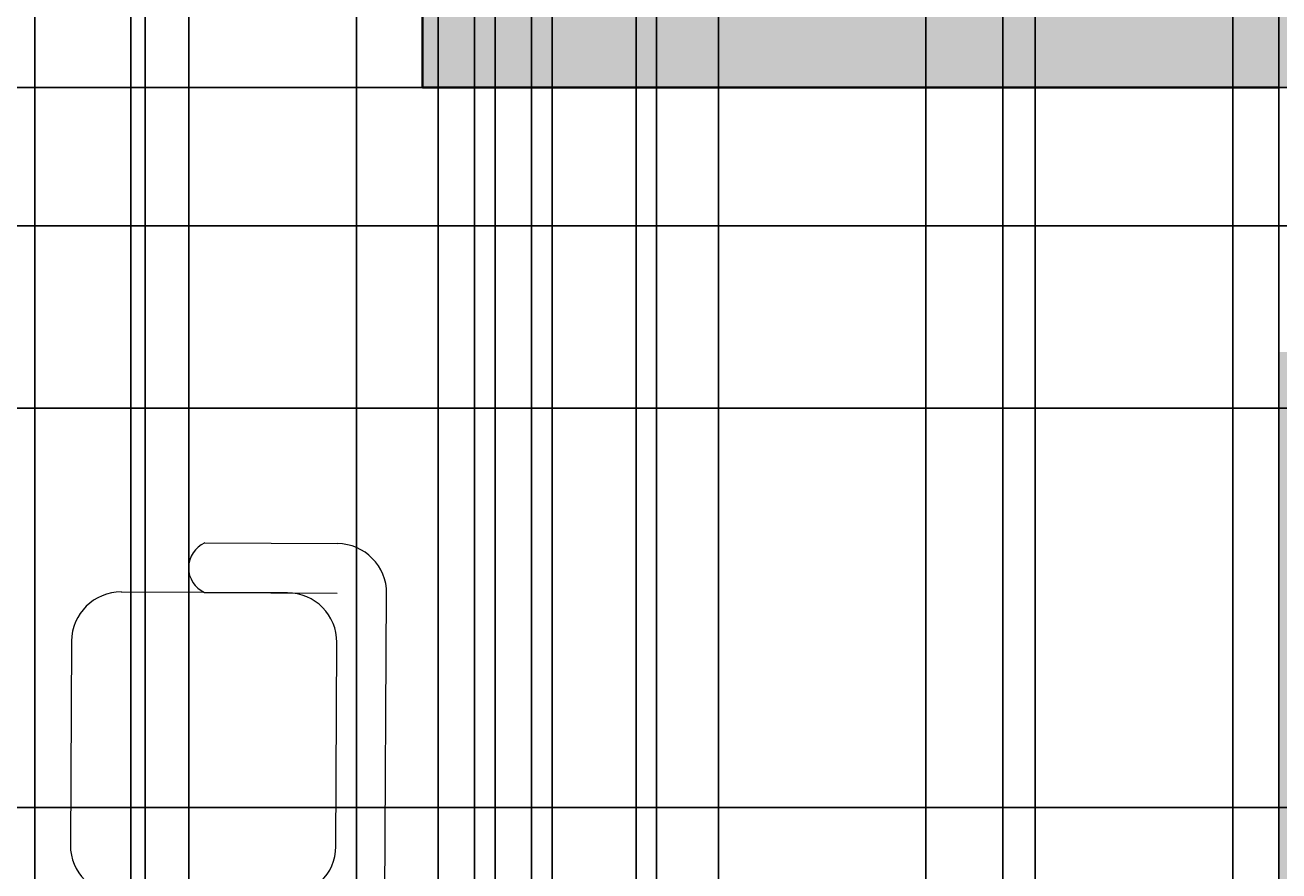
# Model space of a CAD drawing. Units: inches. Extents: x 818 to 1898, y 976 to 2364.
# Tile 37 of 96: x 1391 to 1512, y 1792 to 1873. Entities that reach past the tile are written whole.
import ezdxf

# ---------------------------------------------------------------- set-up
doc = ezdxf.new("R2010")
doc.units = ezdxf.units.IN
doc.header["$LTSCALE"] = 5
doc.header["$MEASUREMENT"] = 0
for name, color, linetype, lineweight in [('A-ANNO-DIMS', 2, 'Continuous', 18), ('A-FURN', 8, 'Continuous', 18), ('A-WALL', 7, 'Continuous', 40)]:
    doc.layers.add(name, color=color, linetype=linetype, lineweight=lineweight)
doc.layers.add('A-WALL-PATT', color=251, linetype='Continuous', lineweight=13, true_color=0x636466)
doc.styles.get("Standard").update_dxf_attribs({"font": 'arial.ttf'})
doc.dimstyles.get("Standard").update_dxf_attribs({"dimtxt": 0.18, "dimasz": 0.18, "dimexe": 0.18, "dimexo": 0.0625, "dimgap": 0.09, "dimtad": 0, "dimtih": 1, "dimtoh": 1, "dimdec": 4, "dimzin": 0, "dimdsep": 46, "dimtxsty": 'Standard', "dimcen": 0.09, "dimadec": 0, "dimazin": 0, "dimtfac": 1, "dimtdec": 4, "dimtofl": 0, "dimtmove": 0, "dimatfit": 3, "dimfxl": 1, "dimtolj": 1, "dimtzin": 0, "dimarcsym": 0})

# ---------------------------------------------------------------- blocks, each defined once
blk = doc.blocks.new('CHAIR-LOUNGE')
for p, q in [((12.94, 38.78), (25.71, 38.71)), ((20.92, 33.97), (4.9, 34.05)), ((12.91, 34.01), (25.69, 33.94)), ((30.3, 4.74), (30.46, 33.92)), ((0.11, 29.31), (0, 9.68)), ((25.56, 9.54), (25.66, 29.17)), ((19.37, 4.79), (3.35, 4.88)), ((4.74, 4.88), (20.76, 4.79)), ((11.36, 4.84), (24.14, 4.77)), ((12.75, 4.84), (25.53, 4.77)), ((12.73, 0.07), (25.5, 0))]:
    blk.add_line(p, q)
for centre, radius, start, end in [((13.99, 36.39), 2.61, 113.7099, 245.6698), ((25.69, 33.94), 4.77, 359.6898, 89.6898), ((4.88, 29.29), 4.77, 89.6898, 179.6898), ((20.89, 29.2), 4.77, 359.6898, 89.6898), ((4.77, 9.65), 4.77, 179.6898, 269.6898), ((20.79, 9.56), 4.77, 269.6898, 359.6898), ((13.7, 2.45), 2.57, 111.7034, 247.6762), ((19.35, 0.03), 4.77, 359.6898, 89.6898), ((25.53, 4.77), 4.77, 269.6898, 359.6898)]:
    blk.add_arc(centre, radius, start, end)
blk = doc.blocks.new('*D61')
at = {"layer": 'A-ANNO-DIMS', "color": 0, "lineweight": -2, "ltscale": 5, "transparency": 16777216}
for p, q in [((1071.73, 1203.03), (1071.73, 2363.87)), ((1071.91, 2363.69), (1250.94, 2363.69)), ((1430.55, 2363.69), (1251.51, 2363.69)), ((1430.73, 1203.03), (1430.73, 2363.87))]:
    blk.add_line(p, q, dxfattribs=at)
at = {"layer": 'A-ANNO-DIMS', "color": 0, "ltscale": 5, "transparency": 16777216}
for points in [[(1071.91, 2363.72), (1071.91, 2363.66), (1071.73, 2363.69)], [(1430.55, 2363.72), (1430.55, 2363.66), (1430.73, 2363.69)]]:
    blk.add_solid(points, dxfattribs=at)
at = {"layer": 'Defpoints', "color": 0, "ltscale": 5, "transparency": 16777216}
for p in [(1430.73, 2363.69), (1071.73, 1202.96), (1430.73, 1202.96)]:
    blk.add_point(p, dxfattribs=at)
at = {"layer": 'A-ANNO-DIMS', "color": 0, "ltscale": 5, "transparency": 16777216, "insert": (1251.23, 2363.69), "char_height": 0.18, "attachment_point": 5}
blk.add_mtext('\\A1;359', dxfattribs=at)
blk = doc.blocks.new('*D64')
at = {"layer": 'A-ANNO-DIMS', "color": 0, "lineweight": -2, "ltscale": 5, "transparency": 16777216}
for p, q in [((1197.73, 1501.14), (1197.73, 2363.87)), ((1197.91, 2363.69), (1313.93, 2363.69)), ((1430.55, 2363.69), (1314.52, 2363.69)), ((1430.73, 1501.14), (1430.73, 2363.87))]:
    blk.add_line(p, q, dxfattribs=at)
at = {"layer": 'A-ANNO-DIMS', "color": 0, "ltscale": 5, "transparency": 16777216}
for points in [[(1197.91, 2363.72), (1197.91, 2363.66), (1197.73, 2363.69)], [(1430.55, 2363.72), (1430.55, 2363.66), (1430.73, 2363.69)]]:
    blk.add_solid(points, dxfattribs=at)
at = {"layer": 'Defpoints', "color": 0, "ltscale": 5, "transparency": 16777216}
for p in [(1430.73, 2363.69), (1197.73, 1501.08), (1430.73, 1501.08)]:
    blk.add_point(p, dxfattribs=at)
at = {"layer": 'A-ANNO-DIMS', "color": 0, "ltscale": 5, "transparency": 16777216, "insert": (1314.23, 2363.69), "char_height": 0.18, "attachment_point": 5}
blk.add_mtext('\\A1;233', dxfattribs=at)
blk = doc.blocks.new('*D85')
at = {"layer": 'A-ANNO-DIMS', "color": 0, "lineweight": -2, "ltscale": 5, "transparency": 16777216}
for p, q in [((1258.79, 2053.08), (1897.92, 2053.08)), ((1897.74, 2052.9), (1897.74, 1876.76)), ((1897.74, 1700.26), (1897.74, 1876.4)), ((1258.79, 1700.08), (1897.92, 1700.08))]:
    blk.add_line(p, q, dxfattribs=at)
at = {"layer": 'A-ANNO-DIMS', "color": 0, "ltscale": 5, "transparency": 16777216}
for points in [[(1897.71, 2052.9), (1897.77, 2052.9), (1897.74, 2053.08)], [(1897.71, 1700.26), (1897.77, 1700.26), (1897.74, 1700.08)]]:
    blk.add_solid(points, dxfattribs=at)
at = {"layer": 'Defpoints', "color": 0, "ltscale": 5, "transparency": 16777216}
for p in [(1258.73, 2053.08), (1897.74, 2053.08), (1258.73, 1700.08)]:
    blk.add_point(p, dxfattribs=at)
at = {"layer": 'A-ANNO-DIMS', "color": 0, "ltscale": 5, "transparency": 16777216, "insert": (1897.74, 1876.58), "char_height": 0.18, "attachment_point": 5}
blk.add_mtext('\\A1;353', dxfattribs=at)
blk = doc.blocks.new('*D98')
at = {"layer": 'A-ANNO-DIMS', "color": 0, "lineweight": -2, "ltscale": 5, "transparency": 16777216}
for p, q in [((1338.54, 1071.12), (1338.54, 2363.87)), ((1338.72, 2363.69), (1364.81, 2363.69)), ((1391.7, 2363.69), (1365.6, 2363.69)), ((1391.88, 1071.12), (1391.88, 2363.87))]:
    blk.add_line(p, q, dxfattribs=at)
at = {"layer": 'A-ANNO-DIMS', "color": 0, "ltscale": 5, "transparency": 16777216}
for points in [[(1338.72, 2363.72), (1338.72, 2363.66), (1338.54, 2363.69)], [(1391.7, 2363.72), (1391.7, 2363.66), (1391.88, 2363.69)]]:
    blk.add_solid(points, dxfattribs=at)
at = {"layer": 'Defpoints', "color": 0, "ltscale": 5, "transparency": 16777216}
for p in [(1391.88, 2363.69), (1338.54, 1071.06), (1391.88, 1071.06)]:
    blk.add_point(p, dxfattribs=at)
at = {"layer": 'A-ANNO-DIMS', "color": 0, "ltscale": 5, "transparency": 16777216, "insert": (1365.21, 2363.69), "char_height": 0.18, "attachment_point": 5}
blk.add_mtext('\\A1;53.33', dxfattribs=at)
blk = doc.blocks.new('*D99')
at = {"layer": 'A-ANNO-DIMS', "color": 0, "lineweight": -2, "ltscale": 5, "transparency": 16777216}
for p, q in [((1391.88, 1071.12), (1391.88, 2363.87)), ((1392.06, 2363.69), (1420.45, 2363.69)), ((1449.64, 2363.69), (1421.24, 2363.69)), ((1449.82, 1071.12), (1449.82, 2363.87))]:
    blk.add_line(p, q, dxfattribs=at)
at = {"layer": 'A-ANNO-DIMS', "color": 0, "ltscale": 5, "transparency": 16777216}
for points in [[(1392.06, 2363.72), (1392.06, 2363.66), (1391.88, 2363.69)], [(1449.64, 2363.72), (1449.64, 2363.66), (1449.82, 2363.69)]]:
    blk.add_solid(points, dxfattribs=at)
at = {"layer": 'Defpoints', "color": 0, "ltscale": 5, "transparency": 16777216}
for p in [(1449.82, 2363.69), (1391.88, 1071.06), (1449.82, 1071.06)]:
    blk.add_point(p, dxfattribs=at)
at = {"layer": 'A-ANNO-DIMS', "color": 0, "ltscale": 5, "transparency": 16777216, "insert": (1420.85, 2363.69), "char_height": 0.18, "attachment_point": 5}
blk.add_mtext('\\A1;57.94', dxfattribs=at)
blk = doc.blocks.new('*D100')
at = {"layer": 'A-ANNO-DIMS', "color": 0, "lineweight": -2, "ltscale": 5, "transparency": 16777216}
for p, q in [((1449.82, 1071.12), (1449.82, 2363.87)), ((1450, 2363.69), (1478.17, 2363.69)), ((1507.12, 2363.69), (1478.95, 2363.69)), ((1507.3, 1071.12), (1507.3, 2363.87))]:
    blk.add_line(p, q, dxfattribs=at)
at = {"layer": 'A-ANNO-DIMS', "color": 0, "ltscale": 5, "transparency": 16777216}
for points in [[(1450, 2363.72), (1450, 2363.66), (1449.82, 2363.69)], [(1507.12, 2363.72), (1507.12, 2363.66), (1507.3, 2363.69)]]:
    blk.add_solid(points, dxfattribs=at)
at = {"layer": 'Defpoints', "color": 0, "ltscale": 5, "transparency": 16777216}
for p in [(1507.3, 2363.69), (1449.82, 1071.06), (1507.3, 1071.06)]:
    blk.add_point(p, dxfattribs=at)
at = {"layer": 'A-ANNO-DIMS', "color": 0, "ltscale": 5, "transparency": 16777216, "insert": (1478.56, 2363.69), "char_height": 0.18, "attachment_point": 5}
blk.add_mtext('\\A1;57.48', dxfattribs=at)
blk = doc.blocks.new('*D101')
at = {"layer": 'A-ANNO-DIMS', "color": 0, "lineweight": -2, "ltscale": 5, "transparency": 16777216}
for p, q in [((1507.3, 1071.12), (1507.3, 2363.87)), ((1507.48, 2363.69), (1536, 2363.69)), ((1565.3, 2363.69), (1536.78, 2363.69)), ((1565.48, 1071.12), (1565.48, 2363.87))]:
    blk.add_line(p, q, dxfattribs=at)
at = {"layer": 'A-ANNO-DIMS', "color": 0, "ltscale": 5, "transparency": 16777216}
for points in [[(1507.48, 2363.72), (1507.48, 2363.66), (1507.3, 2363.69)], [(1565.3, 2363.72), (1565.3, 2363.66), (1565.48, 2363.69)]]:
    blk.add_solid(points, dxfattribs=at)
at = {"layer": 'Defpoints', "color": 0, "ltscale": 5, "transparency": 16777216}
for p in [(1565.48, 2363.69), (1507.3, 1071.06), (1565.48, 1071.06)]:
    blk.add_point(p, dxfattribs=at)
at = {"layer": 'A-ANNO-DIMS', "color": 0, "ltscale": 5, "transparency": 16777216, "insert": (1536.39, 2363.69), "char_height": 0.18, "attachment_point": 5}
blk.add_mtext('\\A1;58.19', dxfattribs=at)
blk = doc.blocks.new('*D120')
at = {"layer": 'A-ANNO-DIMS', "color": 0, "lineweight": -2, "ltscale": 5, "transparency": 16777216}
for p, q in [((1766.29, 1797.72), (818.03, 1797.72)), ((818.21, 1797.54), (818.21, 1757.53)), ((818.21, 1717.17), (818.21, 1757.17)), ((1766.29, 1716.99), (818.03, 1716.99))]:
    blk.add_line(p, q, dxfattribs=at)
at = {"layer": 'A-ANNO-DIMS', "color": 0, "ltscale": 5, "transparency": 16777216}
for points in [[(818.18, 1797.54), (818.24, 1797.54), (818.21, 1797.72)], [(818.18, 1717.17), (818.24, 1717.17), (818.21, 1716.99)]]:
    blk.add_solid(points, dxfattribs=at)
at = {"layer": 'Defpoints', "color": 0, "ltscale": 5, "transparency": 16777216}
for p in [(818.21, 1797.72), (1766.35, 1797.72), (1766.35, 1716.99)]:
    blk.add_point(p, dxfattribs=at)
at = {"layer": 'A-ANNO-DIMS', "color": 0, "ltscale": 5, "transparency": 16777216, "insert": (818.21, 1757.35), "char_height": 0.18, "attachment_point": 5}
blk.add_mtext('\\A1;80.73', dxfattribs=at)
blk = doc.blocks.new('*D121')
at = {"layer": 'A-ANNO-DIMS', "color": 0, "lineweight": -2, "ltscale": 5, "transparency": 16777216}
for p, q in [((1766.29, 1884.2), (818.03, 1884.2)), ((818.21, 1884.02), (818.21, 1841.14)), ((818.21, 1797.9), (818.21, 1840.78)), ((1766.29, 1797.72), (818.03, 1797.72))]:
    blk.add_line(p, q, dxfattribs=at)
at = {"layer": 'A-ANNO-DIMS', "color": 0, "ltscale": 5, "transparency": 16777216}
for points in [[(818.18, 1884.02), (818.24, 1884.02), (818.21, 1884.2)], [(818.18, 1797.9), (818.24, 1797.9), (818.21, 1797.72)]]:
    blk.add_solid(points, dxfattribs=at)
at = {"layer": 'Defpoints', "color": 0, "ltscale": 5, "transparency": 16777216}
for p in [(818.21, 1884.2), (1766.35, 1884.2), (1766.35, 1797.72)]:
    blk.add_point(p, dxfattribs=at)
at = {"layer": 'A-ANNO-DIMS', "color": 0, "ltscale": 5, "transparency": 16777216, "insert": (818.21, 1840.96), "char_height": 0.18, "attachment_point": 5}
blk.add_mtext('\\A1;86.49', dxfattribs=at)
blk = doc.blocks.new('*D162')
at = {"layer": 'A-ANNO-DIMS', "color": 0, "lineweight": -2, "ltscale": 5, "transparency": 16777216}
for p, q in [((1429.16, 1876.08), (818.03, 1876.08)), ((818.21, 1875.9), (818.21, 1871.76)), ((818.21, 1867.26), (818.21, 1871.4)), ((1429.16, 1867.08), (818.03, 1867.08))]:
    blk.add_line(p, q, dxfattribs=at)
at = {"layer": 'A-ANNO-DIMS', "color": 0, "ltscale": 5, "transparency": 16777216}
for points in [[(818.18, 1875.9), (818.24, 1875.9), (818.21, 1876.08)], [(818.18, 1867.26), (818.24, 1867.26), (818.21, 1867.08)]]:
    blk.add_solid(points, dxfattribs=at)
at = {"layer": 'Defpoints', "color": 0, "ltscale": 5, "transparency": 16777216}
for p in [(1429.23, 1876.08), (818.21, 1867.08), (1429.23, 1867.08)]:
    blk.add_point(p, dxfattribs=at)
at = {"layer": 'A-ANNO-DIMS', "color": 0, "ltscale": 5, "transparency": 16777216, "insert": (818.21, 1871.58), "char_height": 0.18, "attachment_point": 5}
blk.add_mtext('\\A1;9', dxfattribs=at)
blk = doc.blocks.new('*D166')
at = {"layer": 'A-ANNO-DIMS', "color": 0, "lineweight": -2, "ltscale": 5, "transparency": 16777216}
for p, q in [((1401.15, 1510.14), (1401.15, 2363.87)), ((1401.33, 2363.69), (1415.54, 2363.69)), ((1430.55, 2363.69), (1416.33, 2363.69)), ((1430.73, 1510.14), (1430.73, 2363.87))]:
    blk.add_line(p, q, dxfattribs=at)
at = {"layer": 'A-ANNO-DIMS', "color": 0, "ltscale": 5, "transparency": 16777216}
for points in [[(1401.33, 2363.72), (1401.33, 2363.66), (1401.15, 2363.69)], [(1430.55, 2363.72), (1430.55, 2363.66), (1430.73, 2363.69)]]:
    blk.add_solid(points, dxfattribs=at)
at = {"layer": 'Defpoints', "color": 0, "ltscale": 5, "transparency": 16777216}
for p in [(1430.73, 2363.69), (1401.15, 1510.08), (1430.73, 1510.08)]:
    blk.add_point(p, dxfattribs=at)
at = {"layer": 'A-ANNO-DIMS', "color": 0, "ltscale": 5, "transparency": 16777216, "insert": (1415.94, 2363.69), "char_height": 0.18, "attachment_point": 5}
blk.add_mtext('\\A1;29.58', dxfattribs=at)
blk = doc.blocks.new('*D169')
at = {"layer": 'A-ANNO-DIMS', "color": 0, "lineweight": -2, "ltscale": 5, "transparency": 16777216}
for p, q in [((1441.73, 1600.14), (1441.73, 2363.87)), ((1441.91, 2363.69), (1459.51, 2363.69)), ((1477.55, 2363.69), (1459.94, 2363.69)), ((1477.73, 1600.14), (1477.73, 2363.87))]:
    blk.add_line(p, q, dxfattribs=at)
at = {"layer": 'A-ANNO-DIMS', "color": 0, "ltscale": 5, "transparency": 16777216}
for points in [[(1441.91, 2363.72), (1441.91, 2363.66), (1441.73, 2363.69)], [(1477.55, 2363.72), (1477.55, 2363.66), (1477.73, 2363.69)]]:
    blk.add_solid(points, dxfattribs=at)
at = {"layer": 'Defpoints', "color": 0, "ltscale": 5, "transparency": 16777216}
for p in [(1477.73, 2363.69), (1441.73, 1600.08), (1477.73, 1600.08)]:
    blk.add_point(p, dxfattribs=at)
at = {"layer": 'A-ANNO-DIMS', "color": 0, "ltscale": 5, "transparency": 16777216, "insert": (1459.73, 2363.69), "char_height": 0.18, "attachment_point": 5}
blk.add_mtext('\\A1;36', dxfattribs=at)
blk = doc.blocks.new('*D191')
at = {"layer": 'A-ANNO-DIMS', "color": 0, "lineweight": -2, "ltscale": 5, "transparency": 16777216}
for p, q in [((1434.23, 1409.11), (1434.23, 2363.87)), ((1434.41, 2363.69), (1435.08, 2363.69)), ((1436.05, 2363.69), (1435.37, 2363.69)), ((1436.23, 1409.11), (1436.23, 2363.87))]:
    blk.add_line(p, q, dxfattribs=at)
at = {"layer": 'A-ANNO-DIMS', "color": 0, "ltscale": 5, "transparency": 16777216}
for points in [[(1434.41, 2363.72), (1434.41, 2363.66), (1434.23, 2363.69)], [(1436.05, 2363.72), (1436.05, 2363.66), (1436.23, 2363.69)]]:
    blk.add_solid(points, dxfattribs=at)
at = {"layer": 'Defpoints', "color": 0, "ltscale": 5, "transparency": 16777216}
for p in [(1436.23, 2363.69), (1434.23, 1409.05), (1436.23, 1409.05)]:
    blk.add_point(p, dxfattribs=at)
at = {"layer": 'A-ANNO-DIMS', "color": 0, "ltscale": 5, "transparency": 16777216, "insert": (1435.23, 2363.69), "char_height": 0.18, "attachment_point": 5}
blk.add_mtext('\\A1;2', dxfattribs=at)
blk = doc.blocks.new('*D196')
at = {"layer": 'A-ANNO-DIMS', "color": 0, "lineweight": -2, "ltscale": 5, "transparency": 16777216}
for p, q in [((1439.73, 1526.73), (1439.73, 2363.87)), ((1439.91, 2363.69), (1448.51, 2363.69)), ((1457.55, 2363.69), (1448.94, 2363.69)), ((1457.73, 1526.73), (1457.73, 2363.87))]:
    blk.add_line(p, q, dxfattribs=at)
at = {"layer": 'A-ANNO-DIMS', "color": 0, "ltscale": 5, "transparency": 16777216}
for points in [[(1439.91, 2363.72), (1439.91, 2363.66), (1439.73, 2363.69)], [(1457.55, 2363.72), (1457.55, 2363.66), (1457.73, 2363.69)]]:
    blk.add_solid(points, dxfattribs=at)
at = {"layer": 'Defpoints', "color": 0, "ltscale": 5, "transparency": 16777216}
for p in [(1457.73, 2363.69), (1439.73, 1526.67), (1457.73, 1526.67)]:
    blk.add_point(p, dxfattribs=at)
at = {"layer": 'A-ANNO-DIMS', "color": 0, "ltscale": 5, "transparency": 16777216, "insert": (1448.73, 2363.69), "char_height": 0.18, "attachment_point": 5}
blk.add_mtext('\\A1;18', dxfattribs=at)
blk = doc.blocks.new('*D215')
at = {"layer": 'A-ANNO-DIMS', "color": 0, "lineweight": -2, "ltscale": 5, "transparency": 16777216}
for p, q in [((1590.66, 1876.08), (818.03, 1876.08)), ((818.21, 1875.9), (818.21, 1781.76)), ((818.21, 1687.26), (818.21, 1781.4)), ((1511.66, 1687.08), (818.03, 1687.08))]:
    blk.add_line(p, q, dxfattribs=at)
at = {"layer": 'A-ANNO-DIMS', "color": 0, "ltscale": 5, "transparency": 16777216}
for points in [[(818.18, 1875.9), (818.24, 1875.9), (818.21, 1876.08)], [(818.18, 1687.26), (818.24, 1687.26), (818.21, 1687.08)]]:
    blk.add_solid(points, dxfattribs=at)
at = {"layer": 'Defpoints', "color": 0, "ltscale": 5, "transparency": 16777216}
for p in [(818.21, 1876.08), (1590.73, 1876.08), (1511.73, 1687.08)]:
    blk.add_point(p, dxfattribs=at)
at = {"layer": 'A-ANNO-DIMS', "color": 0, "ltscale": 5, "transparency": 16777216, "insert": (818.21, 1781.58), "char_height": 0.18, "attachment_point": 5}
blk.add_mtext('\\A1;189', dxfattribs=at)
blk = doc.blocks.new('*D227')
at = {"layer": 'A-ANNO-DIMS', "color": 0, "lineweight": -2, "ltscale": 5, "transparency": 16777216}
for p, q in [((1595.66, 1867.08), (818.03, 1867.08)), ((818.21, 1866.9), (818.21, 1851.81)), ((818.21, 1836.36), (818.21, 1851.45)), ((1594.66, 1836.18), (818.03, 1836.18))]:
    blk.add_line(p, q, dxfattribs=at)
at = {"layer": 'A-ANNO-DIMS', "color": 0, "ltscale": 5, "transparency": 16777216}
for points in [[(818.18, 1866.9), (818.24, 1866.9), (818.21, 1867.08)], [(818.18, 1836.36), (818.24, 1836.36), (818.21, 1836.18)]]:
    blk.add_solid(points, dxfattribs=at)
at = {"layer": 'Defpoints', "color": 0, "ltscale": 5, "transparency": 16777216}
for p in [(818.21, 1867.08), (1595.73, 1867.08), (1594.73, 1836.18)]:
    blk.add_point(p, dxfattribs=at)
at = {"layer": 'A-ANNO-DIMS', "color": 0, "ltscale": 5, "transparency": 16777216, "insert": (818.21, 1851.63), "char_height": 0.18, "attachment_point": 5}
blk.add_mtext('\\A1;30.894', dxfattribs=at)
blk = doc.blocks.new('*D231')
at = {"layer": 'A-ANNO-DIMS', "color": 0, "lineweight": -2, "ltscale": 5, "transparency": 16777216}
for p, q in [((1303.93, 1952.98), (1303.93, 975.66)), ((1402.52, 1952.98), (1402.52, 975.66)), ((1304.11, 975.84), (1352.83, 975.84)), ((1402.34, 975.84), (1353.62, 975.84))]:
    blk.add_line(p, q, dxfattribs=at)
at = {"layer": 'A-ANNO-DIMS', "color": 0, "ltscale": 5, "transparency": 16777216}
for points in [[(1304.11, 975.87), (1304.11, 975.81), (1303.93, 975.84)], [(1402.34, 975.87), (1402.34, 975.81), (1402.52, 975.84)]]:
    blk.add_solid(points, dxfattribs=at)
at = {"layer": 'Defpoints', "color": 0, "ltscale": 5, "transparency": 16777216}
for p in [(1303.93, 1953.04), (1402.52, 1953.04), (1402.52, 975.84)]:
    blk.add_point(p, dxfattribs=at)
at = {"layer": 'A-ANNO-DIMS', "color": 0, "ltscale": 5, "transparency": 16777216, "insert": (1353.22, 975.84), "char_height": 0.18, "attachment_point": 5}
blk.add_mtext('\\A1;98.59', dxfattribs=at)
blk = doc.blocks.new('*D242')
at = {"layer": 'A-ANNO-DIMS', "color": 0, "lineweight": -2, "ltscale": 5, "transparency": 16777216}
for p, q in [((1488.26, 1948.6), (1488.26, 975.66)), ((1513.23, 1948.6), (1513.23, 975.66)), ((1488.44, 975.84), (1500.35, 975.84)), ((1513.05, 975.84), (1501.14, 975.84))]:
    blk.add_line(p, q, dxfattribs=at)
at = {"layer": 'A-ANNO-DIMS', "color": 0, "ltscale": 5, "transparency": 16777216}
for points in [[(1488.44, 975.87), (1488.44, 975.81), (1488.26, 975.84)], [(1513.05, 975.87), (1513.05, 975.81), (1513.23, 975.84)]]:
    blk.add_solid(points, dxfattribs=at)
at = {"layer": 'Defpoints', "color": 0, "ltscale": 5, "transparency": 16777216}
for p in [(1488.26, 1948.66), (1513.23, 1948.66), (1513.23, 975.84)]:
    blk.add_point(p, dxfattribs=at)
at = {"layer": 'A-ANNO-DIMS', "color": 0, "ltscale": 5, "transparency": 16777216, "insert": (1500.74, 975.84), "char_height": 0.18, "attachment_point": 5}
blk.add_mtext('\\A1;24.97', dxfattribs=at)
blk = doc.blocks.new('*D243')
at = {"layer": 'A-ANNO-DIMS', "color": 0, "lineweight": -2, "ltscale": 5, "transparency": 16777216}
for p, q in [((1451.77, 2020.02), (1451.77, 975.66)), ((1590.73, 2020.02), (1590.73, 975.66)), ((1451.95, 975.84), (1520.79, 975.84)), ((1590.55, 975.84), (1521.7, 975.84))]:
    blk.add_line(p, q, dxfattribs=at)
at = {"layer": 'A-ANNO-DIMS', "color": 0, "ltscale": 5, "transparency": 16777216}
for points in [[(1451.95, 975.87), (1451.95, 975.81), (1451.77, 975.84)], [(1590.55, 975.87), (1590.55, 975.81), (1590.73, 975.84)]]:
    blk.add_solid(points, dxfattribs=at)
at = {"layer": 'Defpoints', "color": 0, "ltscale": 5, "transparency": 16777216}
for p in [(1451.77, 2020.08), (1590.73, 2020.08), (1590.73, 975.84)]:
    blk.add_point(p, dxfattribs=at)
at = {"layer": 'A-ANNO-DIMS', "color": 0, "ltscale": 5, "transparency": 16777216, "insert": (1521.25, 975.84), "char_height": 0.18, "attachment_point": 5}
blk.add_mtext('\\A1;138.96', dxfattribs=at)
blk = doc.blocks.new('*D253')
at = {"layer": 'A-ANNO-DIMS', "color": 0, "lineweight": -2, "ltscale": 5, "transparency": 16777216}
for p, q in [((1485.12, 2053.02), (1485.12, 975.66)), ((1538.52, 2053.02), (1538.52, 975.66)), ((1485.3, 975.84), (1511.42, 975.84)), ((1538.34, 975.84), (1512.21, 975.84))]:
    blk.add_line(p, q, dxfattribs=at)
at = {"layer": 'A-ANNO-DIMS', "color": 0, "ltscale": 5, "transparency": 16777216}
for points in [[(1485.3, 975.87), (1485.3, 975.81), (1485.12, 975.84)], [(1538.34, 975.87), (1538.34, 975.81), (1538.52, 975.84)]]:
    blk.add_solid(points, dxfattribs=at)
at = {"layer": 'Defpoints', "color": 0, "ltscale": 5, "transparency": 16777216}
for p in [(1485.12, 2053.08), (1538.52, 2053.08), (1538.52, 975.84)]:
    blk.add_point(p, dxfattribs=at)
at = {"layer": 'A-ANNO-DIMS', "color": 0, "ltscale": 5, "transparency": 16777216, "insert": (1511.82, 975.84), "char_height": 0.18, "attachment_point": 5}
blk.add_mtext('\\A1;53.39', dxfattribs=at)
blk = doc.blocks.new('*D273')
at = {"layer": 'A-ANNO-DIMS', "color": 0, "lineweight": -2, "ltscale": 5, "transparency": 16777216}
for p, q in [((1406.73, 1587.48), (1406.73, 2363.87)), ((1406.91, 2363.69), (1418.51, 2363.69)), ((1430.55, 2363.69), (1418.95, 2363.69)), ((1430.73, 1587.48), (1430.73, 2363.87))]:
    blk.add_line(p, q, dxfattribs=at)
at = {"layer": 'A-ANNO-DIMS', "color": 0, "ltscale": 5, "transparency": 16777216}
for points in [[(1406.91, 2363.72), (1406.91, 2363.66), (1406.73, 2363.69)], [(1430.55, 2363.72), (1430.55, 2363.66), (1430.73, 2363.69)]]:
    blk.add_solid(points, dxfattribs=at)
at = {"layer": 'Defpoints', "color": 0, "ltscale": 5, "transparency": 16777216}
for p in [(1430.73, 2363.69), (1406.73, 1587.42), (1430.73, 1587.42)]:
    blk.add_point(p, dxfattribs=at)
at = {"layer": 'A-ANNO-DIMS', "color": 0, "ltscale": 5, "transparency": 16777216, "insert": (1418.73, 2363.69), "char_height": 0.18, "attachment_point": 5}
blk.add_mtext('\\A1;24', dxfattribs=at)
blk = doc.blocks.new('*D275')
at = {"layer": 'A-ANNO-DIMS', "color": 0, "lineweight": -2, "ltscale": 5, "transparency": 16777216}
for p, q in [((1377.84, 1897.87), (1897.92, 1897.87)), ((1897.74, 1897.69), (1897.74, 1875.99)), ((1897.74, 1853.93), (1897.74, 1875.63)), ((1377.84, 1853.75), (1897.92, 1853.75))]:
    blk.add_line(p, q, dxfattribs=at)
at = {"layer": 'A-ANNO-DIMS', "color": 0, "ltscale": 5, "transparency": 16777216}
for points in [[(1897.71, 1897.69), (1897.77, 1897.69), (1897.74, 1897.87)], [(1897.71, 1853.93), (1897.77, 1853.93), (1897.74, 1853.75)]]:
    blk.add_solid(points, dxfattribs=at)
at = {"layer": 'Defpoints', "color": 0, "ltscale": 5, "transparency": 16777216}
for p in [(1377.78, 1897.87), (1897.74, 1897.87), (1377.78, 1853.75)]:
    blk.add_point(p, dxfattribs=at)
at = {"layer": 'A-ANNO-DIMS', "color": 0, "ltscale": 5, "transparency": 16777216, "insert": (1897.74, 1875.81), "char_height": 0.18, "attachment_point": 5}
blk.add_mtext('\\A1;44.12', dxfattribs=at)
blk = doc.blocks.new('*D282')
at = {"layer": 'A-ANNO-DIMS', "color": 0, "lineweight": -2, "ltscale": 5, "transparency": 16777216}
for p, q in [((1422.08, 2081.19), (1897.92, 2081.19)), ((1897.74, 2081.01), (1897.74, 1884.32)), ((1897.74, 1687.26), (1897.74, 1883.95)), ((1463.79, 1687.08), (1897.92, 1687.08))]:
    blk.add_line(p, q, dxfattribs=at)
at = {"layer": 'A-ANNO-DIMS', "color": 0, "ltscale": 5, "transparency": 16777216}
for points in [[(1897.71, 2081.01), (1897.77, 2081.01), (1897.74, 2081.19)], [(1897.71, 1687.26), (1897.77, 1687.26), (1897.74, 1687.08)]]:
    blk.add_solid(points, dxfattribs=at)
at = {"layer": 'Defpoints', "color": 0, "ltscale": 5, "transparency": 16777216}
for p in [(1422.02, 2081.19), (1897.74, 2081.19), (1463.73, 1687.08)]:
    blk.add_point(p, dxfattribs=at)
at = {"layer": 'A-ANNO-DIMS', "color": 0, "ltscale": 5, "transparency": 16777216, "insert": (1897.74, 1884.13), "char_height": 0.18, "attachment_point": 5}
blk.add_mtext('\\A1;394.1', dxfattribs=at)
blk = doc.blocks.new('*D288')
at = {"layer": 'A-ANNO-DIMS', "color": 0, "lineweight": -2, "ltscale": 5, "transparency": 16777216}
for p, q in [((1422.88, 1742.67), (1422.88, 2363.87)), ((1423.06, 2363.69), (1466.91, 2363.69)), ((1511.55, 2363.69), (1467.69, 2363.69)), ((1511.73, 1716.11), (1511.73, 2363.87))]:
    blk.add_line(p, q, dxfattribs=at)
at = {"layer": 'A-ANNO-DIMS', "color": 0, "ltscale": 5, "transparency": 16777216}
for points in [[(1423.06, 2363.72), (1423.06, 2363.66), (1422.88, 2363.69)], [(1511.55, 2363.72), (1511.55, 2363.66), (1511.73, 2363.69)]]:
    blk.add_solid(points, dxfattribs=at)
at = {"layer": 'Defpoints', "color": 0, "ltscale": 5, "transparency": 16777216}
for p in [(1511.73, 2363.69), (1422.88, 1742.61), (1511.73, 1716.05)]:
    blk.add_point(p, dxfattribs=at)
at = {"layer": 'A-ANNO-DIMS', "color": 0, "ltscale": 5, "transparency": 16777216, "insert": (1467.3, 2363.69), "char_height": 0.18, "attachment_point": 5}
blk.add_mtext('\\A1;88.85', dxfattribs=at)

msp = doc.modelspace()

# ---------------------------------------------------------------- hatches: boundary and pattern name
at = {"layer": 'A-WALL-PATT', "ltscale": 5}
h = msp.add_hatch(color=256, dxfattribs=at)
h.dxf.hatch_style = 1
h.paths.add_polyline_path([(1267.7252, 1928.9218), (1258.7251, 1928.9218), (1258.7251, 1913.6401), (1250.3029, 1913.6401), (1250.3029, 1878.3919), (1258.7251, 1878.3919), (1258.7251, 1862.9652), (1267.7252, 1862.9652)])
h.paths.add_polyline_path([(1267.7252, 1814.9652), (1258.7251, 1814.9652), (1258.7251, 1755.3321), (1267.7252, 1755.3321)])
h.paths.add_polyline_path([(1463.7251, 1696.0782), (1267.7252, 1696.0782), (1267.7252, 1707.3321), (1258.7251, 1707.3321), (1258.7251, 1700.0782), (1251.9333, 1700.0782), (1251.9333, 1687.0782), (1463.7251, 1687.0782)])
h.paths.add_polyline_path([(1714.7252, 1717.3178), (1705.7252, 1717.3178), (1705.7252, 1696.0782), (1599.7252, 1696.0782), (1599.7252, 1790.0782), (1705.7252, 1790.0782), (1705.7252, 1785.6125), (1714.7252, 1785.6125), (1714.7252, 1827.2125), (1705.7252, 1827.2125), (1705.7252, 1802.0782), (1599.7252, 1802.0782), (1599.7252, 1867.0782), (1705.7252, 1867.0782), (1705.7252, 1857.2125), (1714.7252, 1857.2125), (1714.7252, 1930.0316), (1741.8409, 1930.0316), (1741.8409, 1935.0316), (1714.7252, 1935.0316), (1714.7252, 1957.0338), (1741.8409, 1957.0338), (1741.8409, 1962.0338), (1714.7252, 1962.0338), (1705.7252, 1962.0338), (1705.7252, 1948.0782), (1599.7252, 1948.0782), (1599.7252, 1981.0782), (1590.7251, 1981.0782), (1590.7251, 1941.0782), (1620.7252, 1941.0782), (1705.7252, 1941.0782), (1705.7252, 1876.0782), (1599.7252, 1876.0782), (1599.7252, 1911.0782), (1590.7251, 1911.0782), (1590.7251, 1876.0782), (1429.2251, 1876.0782), (1429.2251, 1867.0782), (1511.7251, 1867.0782), (1528.593, 1867.0782), (1595.7251, 1867.0782), (1595.7251, 1773.0782), (1520.7252, 1773.0782), (1520.7252, 1837.5823), (1532.593, 1837.5823), (1532.593, 1867.0782), (1528.593, 1867.0782), (1528.593, 1841.5823), (1511.7251, 1841.5823), (1511.7251, 1744.9714), (1520.7252, 1744.9714), (1520.7252, 1761.0782), (1595.7251, 1761.0782), (1595.7251, 1696.0782), (1520.7252, 1696.0782), (1520.7252, 1716.0454), (1511.7251, 1716.0454), (1511.7251, 1696.0782), (1511.7251, 1687.0782), (1714.7252, 1687.0782)])
h.paths.add_polyline_path([(1714.7252, 2053.0782), (1714.7252, 2081.1881), (1709.7252, 2081.1881), (1709.7252, 2053.0782), (1681.6446, 2053.0782), (1681.6446, 2081.1881), (1676.6446, 2081.1881), (1676.6446, 2053.0782), (1538.5155, 2053.0782), (1538.5155, 2044.0782), (1590.7251, 2044.0782), (1590.7251, 2011.0782), (1599.7252, 2011.0782), (1599.7252, 2044.0782), (1705.7252, 2044.0782), (1705.7252, 2014.5114), (1714.7252, 2014.5114)])
h.paths.add_polyline_path([(1485.1216, 2053.0782), (1422.02, 2053.0782), (1422.02, 2081.1881), (1413.02, 2081.1881), (1413.02, 2053.0782), (1399.6356, 2053.0782), (1399.6356, 2081.1881), (1390.6356, 2081.1881), (1390.6356, 2053.0782), (1388.0315, 2053.0782), (1388.0315, 2044.0782), (1416.2743, 2044.0782), (1485.1216, 2044.0782)])
h.paths.add_polyline_path([(1330.305, 2053.0782), (1258.7251, 2053.0782), (1258.7251, 2019.2871), (1267.7252, 2019.2871), (1267.7252, 2044.0782), (1330.305, 2044.0782)])
h.paths.add_polyline_path([(1258.7251, 2053.0782), (1214.6577, 2053.0782), (1214.6577, 2044.0782), (1258.7251, 2044.0782)])
h.paths.add_polyline_path([(1214.6577, 2053.0782), (1180.349, 2053.0782), (1180.349, 2044.0782), (1214.6577, 2044.0782)])
h.paths.add_polyline_path([(1714.7252, 1639.5782), (1741.8409, 1639.5782), (1741.8409, 1643.5782), (1714.7252, 1643.5782), (1714.7252, 1649.9029), (1705.7252, 1649.9029), (1705.7252, 1600.0782), (1477.7251, 1600.0782), (1477.7251, 1591.0782), (1520.7252, 1591.0782), (1616.7252, 1591.0782), (1616.7252, 1416.6857), (1622.7252, 1416.6857), (1622.7252, 1463.0782), (1624.7252, 1463.0782), (1624.7252, 1467.0782), (1622.7252, 1467.0782), (1622.7252, 1591.0782), (1705.7252, 1591.0782), (1705.7252, 1545.0782), (1714.7252, 1545.0782), (1741.8409, 1545.0782), (1741.8409, 1549.0782), (1714.7252, 1549.0782), (1714.7252, 1593.9175), (1737.8409, 1593.9175), (1737.8409, 1597.9175), (1714.7252, 1597.9175)])
h.paths.add_polyline_path([(1674.9024, 2060.7419), (1714.7045, 2060.7419), (1714.7045, 2073.1061), (1674.9024, 2073.1061)], flags=25)
h.paths.add_polyline_path([(1394.5468, 2061.6618), (1422.2344, 2061.6618), (1422.2344, 2074.0261), (1394.5468, 2074.0261)], flags=24)

# ---------------------------------------------------------------- linework, layer by layer
at = {"layer": 'A-WALL'}
for p, q in [((1429.2251, 1876.0782), (1429.2251, 1867.0782)), ((1429.2251, 1867.0782), (1511.7251, 1867.0782))]:
    msp.add_line(p, q, dxfattribs=at)

# ---------------------------------------------------------------- block references
at = {"layer": 'A-FURN'}
msp.add_blockref('CHAIR-LOUNGE', (1395.3178, 1784.4245), dxfattribs=at)

# ---------------------------------------------------------------- dimensions: what is measured, and where the dimension line sits
at = {"layer": 'A-ANNO-DIMS', "ltscale": 5}
for base, p1, p2, override, picture, middle in [((1430.7251, 2363.6929), (1071.7251, 1202.9642), (1430.7251, 1202.9642), {"dimdec": 0, "dimlfac": 1, "dimrnd": 0, "dimzin": 0, "dimdsep": 46, "dimlunit": 2}, '*D61', (1251.2251, 2363.6929)), ((1430.7251, 2363.6929), (1197.7251, 1501.0782), (1430.7251, 1501.0782), {"dimdec": 0, "dimlfac": 1, "dimrnd": 0, "dimzin": 0, "dimdsep": 46, "dimlunit": 2}, '*D64', (1314.2251, 2363.6929)), ((1391.8757, 2363.6929), (1338.5412, 1071.0552), (1391.8757, 1071.0552), {"dimdec": 2, "dimlfac": 1, "dimrnd": 0, "dimzin": 0, "dimdsep": 46, "dimlunit": 2}, '*D98', (1365.2084, 2363.6929)), ((1449.8196, 2363.6929), (1391.8757, 1071.0552), (1449.8196, 1071.0552), {"dimdec": 2, "dimlfac": 1, "dimrnd": 0, "dimzin": 0, "dimdsep": 46, "dimlunit": 2}, '*D99', (1420.8477, 2363.6929)), ((1430.7251, 2363.6929), (1401.1463, 1510.0782), (1430.7251, 1510.0782), {"dimdec": 2, "dimlfac": 1, "dimrnd": 0, "dimzin": 0, "dimdsep": 46, "dimlunit": 2}, '*D166', (1415.9357, 2363.6929)), ((1430.7251, 2363.6929), (1406.7251, 1587.4164), (1430.7251, 1587.4164), {"dimdec": 0, "dimlfac": 1, "dimrnd": 0, "dimzin": 0, "dimdsep": 46, "dimlunit": 2}, '*D273', (1418.7251, 2363.6929)), ((1511.7251, 2363.6929), (1422.8756, 1742.6113), (1511.7251, 1716.0454), {"dimdec": 2, "dimlfac": 1, "dimrnd": 0, "dimzin": 0, "dimdsep": 46, "dimlunit": 2}, '*D288', (1467.3004, 2363.6929)), ((1436.2251, 2363.6929), (1434.2251, 1409.0522), (1436.2251, 1409.0522), {"dimdec": 0, "dimlfac": 1, "dimrnd": 0, "dimzin": 0, "dimdsep": 46, "dimlunit": 2}, '*D191', (1435.2251, 2363.6929)), ((1457.7251, 2363.6929), (1439.7251, 1526.6712), (1457.7251, 1526.6712), {"dimdec": 0, "dimlfac": 1, "dimrnd": 0, "dimzin": 0, "dimdsep": 46, "dimlunit": 2}, '*D196', (1448.7251, 2363.6929)), ((1477.7251, 2363.6929), (1441.7251, 1600.0782), (1477.7251, 1600.0782), {"dimdec": 0, "dimlfac": 1, "dimrnd": 0, "dimzin": 0, "dimdsep": 46, "dimlunit": 2}, '*D169', (1459.7251, 2363.6929)), ((1507.2982, 2363.6929), (1449.8196, 1071.0552), (1507.2982, 1071.0552), {"dimdec": 2, "dimlfac": 1, "dimrnd": 0, "dimzin": 0, "dimdsep": 46, "dimlunit": 2}, '*D100', (1478.5589, 2363.6929)), ((1565.4835, 2363.6929), (1507.2982, 1071.0552), (1565.4835, 1071.0552), {"dimdec": 2, "dimlfac": 1, "dimrnd": 0, "dimzin": 0, "dimdsep": 46, "dimlunit": 2}, '*D101', (1536.3908, 2363.6929)), ((1538.5155, 975.8433), (1485.1216, 2053.0782), (1538.5155, 2053.0782), {"dimdec": 2, "dimlfac": 1, "dimrnd": 0, "dimzin": 0, "dimdsep": 46, "dimlunit": 2}, '*D253', (1511.8185, 975.8433)), ((1590.7251, 975.8433), (1451.7698, 2020.0782), (1590.7251, 2020.0782), {"dimdec": 2, "dimlfac": 1, "dimrnd": 0, "dimzin": 0, "dimdsep": 46, "dimlunit": 2}, '*D243', (1521.2475, 975.8433)), ((1402.518, 975.8433), (1303.9314, 1953.0408), (1402.518, 1953.0408), {"dimdec": 2, "dimlfac": 1, "dimrnd": 0, "dimzin": 0, "dimdsep": 46, "dimlunit": 2}, '*D231', (1353.2247, 975.8433)), ((1513.2306, 975.8433), (1488.2586, 1948.6602), (1513.2306, 1948.6602), {"dimdec": 2, "dimlfac": 1, "dimrnd": 0, "dimzin": 0, "dimdsep": 46, "dimlunit": 2}, '*D242', (1500.7446, 975.8433))]:
    dim = msp.add_linear_dim(base=base, p1=p1, p2=p2, dimstyle='Standard', override=override, dxfattribs=at)
    dim.commit()
    dim.dimension.update_dxf_attribs({"geometry": picture, "text_midpoint": middle})
for base, p1, p2, override, picture, middle in [((1897.736, 2081.1881), (1463.7251, 1687.0782), (1422.02, 2081.1881), {"dimdec": 1, "dimlfac": 1, "dimrnd": 0, "dimzin": 0, "dimdsep": 46, "dimlunit": 2}, '*D282', (1897.736, 1884.1332)), ((1897.736, 2053.0782), (1258.7251, 1700.0782), (1258.7251, 2053.0782), {"dimdec": 0, "dimlfac": 1, "dimrnd": 0, "dimzin": 0, "dimdsep": 46, "dimlunit": 2}, '*D85', (1897.736, 1876.5782)), ((1897.736, 1897.8663), (1377.7791, 1853.7496), (1377.7791, 1897.8663), {"dimdec": 2, "dimlfac": 1, "dimrnd": 0, "dimzin": 0, "dimdsep": 46, "dimlunit": 2}, '*D275', (1897.736, 1875.808)), ((818.2059, 1884.2031), (1766.3524, 1797.7165), (1766.3524, 1884.2031), {"dimdec": 2, "dimlfac": 1, "dimrnd": 0, "dimzin": 0, "dimdsep": 46, "dimlunit": 2}, '*D121', (818.2059, 1840.9598)), ((818.2059, 1876.0782), (1511.7251, 1687.0782), (1590.7251, 1876.0782), {"dimdec": 0, "dimlfac": 1, "dimrnd": 0, "dimzin": 0, "dimdsep": 46, "dimlunit": 2}, '*D215', (818.2059, 1781.5782)), ((818.2059, 1867.0782), (1429.2251, 1876.0782), (1429.2251, 1867.0782), {"dimdec": 0, "dimlfac": 1, "dimrnd": 0, "dimzin": 0, "dimdsep": 46, "dimlunit": 2}, '*D162', (818.2059, 1871.5782)), ((818.2059, 1867.0782), (1594.7251, 1836.1844), (1595.7251, 1867.0782), {"dimdec": 3, "dimlfac": 1, "dimrnd": 0, "dimzin": 0, "dimdsep": 46, "dimlunit": 2}, '*D227', (818.2059, 1851.6313)), ((818.2059, 1797.7165), (1766.3524, 1716.9866), (1766.3524, 1797.7165), {"dimdec": 2, "dimlfac": 1, "dimrnd": 0, "dimzin": 0, "dimdsep": 46, "dimlunit": 2}, '*D120', (818.2059, 1757.3516))]:
    dim = msp.add_linear_dim(base=base, p1=p1, p2=p2, angle=90, dimstyle='Standard', override=override, dxfattribs=at)
    dim.commit()
    dim.dimension.update_dxf_attribs({"geometry": picture, "text_midpoint": middle})

doc.saveas('drawing.dxf')
